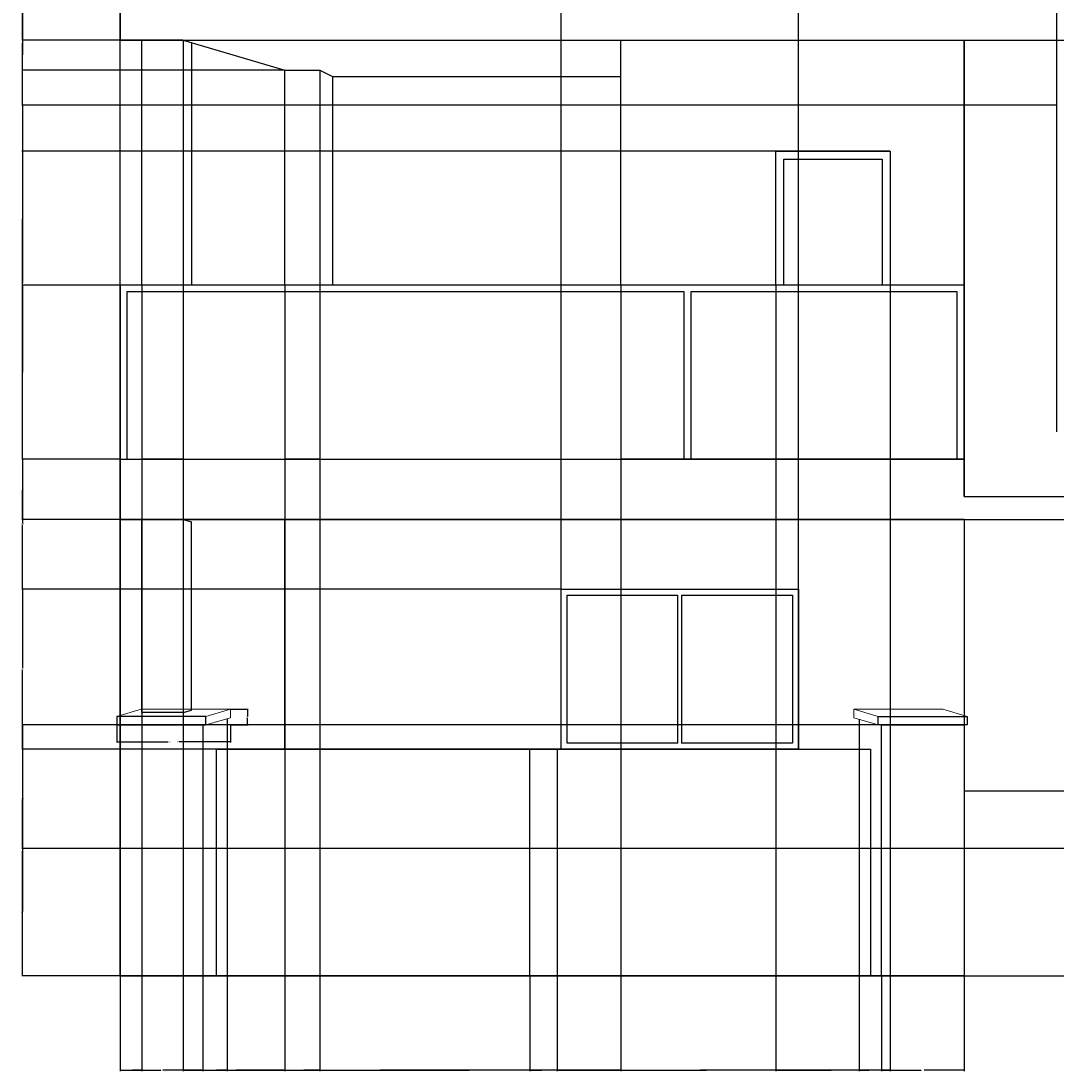
# Model space of a CAD drawing. Units: feet. Extents: x 2926 to 4178, y 965 to 1469.
# Tile 7 of 9: x 3641 to 3913, y 965 to 1241. Entities that reach past the tile are written whole.
import ezdxf

# ---------------------------------------------------------------- set-up
doc = ezdxf.new("R2010")
doc.units = ezdxf.units.FT
for name, color, linetype, lineweight in [('A-ANNO-DIMS', 2, 'Continuous', 18), ('A-ELEV', 7, 'Continuous', 25), ('A-ELEV-DETL', 8, 'Continuous', 18)]:
    doc.layers.add(name, color=color, linetype=linetype, lineweight=lineweight)
doc.styles.get("Standard").update_dxf_attribs({"font": 'arial.ttf'})
doc.dimstyles.get("Standard").update_dxf_attribs({"dimtxt": 0.18, "dimasz": 0.18, "dimexe": 0.18, "dimexo": 0.0625, "dimgap": 0.09, "dimtad": 0, "dimtih": 1, "dimtoh": 1, "dimdec": 1, "dimzin": 0, "dimdsep": 46, "dimlunit": 3, "dimtxsty": 'Standard', "dimcen": 0.09, "dimadec": 0, "dimazin": 0, "dimtfac": 1, "dimtdec": 1, "dimtofl": 0, "dimtmove": 0, "dimatfit": 3, "dimfxl": 1, "dimtolj": 1, "dimtzin": 0, "dimarcsym": 0})

# ---------------------------------------------------------------- blocks, each defined once
blk = doc.blocks.new('PILLAR-CAP-B')
for p, q in [((0, 2.25), (6.42, 4.14)), ((29.85, 4.14), (6.42, 4.14)), ((23.43, 2.25), (29.85, 4.14)), ((29.85, 1.89), (29.85, 4.14)), ((23.43, 0), (29.85, 1.89))]:
    blk.add_line(p, q)
blk = doc.blocks.new('*D8')
at = {"layer": 'A-ANNO-DIMS', "color": 0, "lineweight": -2, "transparency": 16777216}
for p, q in [((3666.26, 1056.26), (3666.26, 1051.66)), ((3696.11, 1056.26), (3696.11, 1051.66)), ((3666.44, 1051.84), (3679.78, 1051.84)), ((3695.93, 1051.84), (3682.59, 1051.84))]:
    blk.add_line(p, q, dxfattribs=at)
at = {"layer": 'A-ANNO-DIMS', "color": 0, "transparency": 16777216}
for points in [[(3666.44, 1051.87), (3666.44, 1051.81), (3666.26, 1051.84)], [(3695.93, 1051.87), (3695.93, 1051.81), (3696.11, 1051.84)]]:
    blk.add_solid(points, dxfattribs=at)
at = {"layer": 'Defpoints', "color": 0, "transparency": 16777216}
for p in [(3666.26, 1056.32), (3696.11, 1056.32), (3696.11, 1051.84)]:
    blk.add_point(p, dxfattribs=at)
at = {"layer": 'A-ANNO-DIMS', "color": 0, "transparency": 16777216, "insert": (3681.19, 1051.84), "char_height": 0.18, "attachment_point": 5}
blk.add_mtext('\\A1;PILLAR CAP B 30 TYP.', dxfattribs=at)
blk = doc.blocks.new('*D9')
at = {"layer": 'A-ANNO-DIMS', "color": 0, "lineweight": -2, "transparency": 16777216}
for p, q in [((3696.17, 1060.46), (3700.77, 1060.46)), ((3700.59, 1060.28), (3700.59, 1058.57)), ((3700.59, 1056.5), (3700.59, 1058.21)), ((3696.17, 1056.32), (3700.77, 1056.32))]:
    blk.add_line(p, q, dxfattribs=at)
at = {"layer": 'A-ANNO-DIMS', "color": 0, "transparency": 16777216}
for points in [[(3700.56, 1060.28), (3700.62, 1060.28), (3700.59, 1060.46)], [(3700.56, 1056.5), (3700.62, 1056.5), (3700.59, 1056.32)]]:
    blk.add_solid(points, dxfattribs=at)
at = {"layer": 'Defpoints', "color": 0, "transparency": 16777216}
for p in [(3696.11, 1060.46), (3700.59, 1060.46), (3696.11, 1056.32)]:
    blk.add_point(p, dxfattribs=at)
at = {"layer": 'A-ANNO-DIMS', "color": 0, "transparency": 16777216, "insert": (3700.59, 1058.39), "char_height": 0.18, "attachment_point": 5}
blk.add_mtext('\\A1;4 TYP.', dxfattribs=at)
blk = doc.blocks.new('*D76')
at = {"layer": 'A-ANNO-DIMS', "color": 0, "lineweight": -2, "transparency": 16777216}
for p, q in [((4050.56, 1023.86), (3641.28, 1023.86)), ((3641.46, 1023.68), (3641.46, 1007.27)), ((3641.46, 990.5), (3641.46, 1006.91)), ((3667.05, 990.32), (3641.28, 990.32))]:
    blk.add_line(p, q, dxfattribs=at)
at = {"layer": 'A-ANNO-DIMS', "color": 0, "transparency": 16777216}
for points in [[(3641.43, 1023.68), (3641.49, 1023.68), (3641.46, 1023.86)], [(3641.43, 990.5), (3641.49, 990.5), (3641.46, 990.32)]]:
    blk.add_solid(points, dxfattribs=at)
at = {"layer": 'Defpoints', "color": 0, "transparency": 16777216}
for p in [(3641.46, 1023.86), (4050.62, 1023.86), (3667.11, 990.32)]:
    blk.add_point(p, dxfattribs=at)
at = {"layer": 'A-ANNO-DIMS', "color": 0, "transparency": 16777216, "insert": (3641.46, 1007.09), "char_height": 0.18, "attachment_point": 5}
blk.add_mtext('\\A1;33.53', dxfattribs=at)
blk = doc.blocks.new('*D77')
at = {"layer": 'A-ANNO-DIMS', "color": 0, "lineweight": -2, "transparency": 16777216}
for p, q in [((3782.96, 1049.98), (3641.28, 1049.98)), ((3641.46, 1049.8), (3641.46, 1037.1)), ((3641.46, 1024.04), (3641.46, 1036.74)), ((4050.56, 1023.86), (3641.28, 1023.86))]:
    blk.add_line(p, q, dxfattribs=at)
at = {"layer": 'A-ANNO-DIMS', "color": 0, "transparency": 16777216}
for points in [[(3641.43, 1049.8), (3641.49, 1049.8), (3641.46, 1049.98)], [(3641.43, 1024.04), (3641.49, 1024.04), (3641.46, 1023.86)]]:
    blk.add_solid(points, dxfattribs=at)
at = {"layer": 'Defpoints', "color": 0, "transparency": 16777216}
for p in [(3641.46, 1049.98), (3783.02, 1049.98), (4050.62, 1023.86)]:
    blk.add_point(p, dxfattribs=at)
at = {"layer": 'A-ANNO-DIMS', "color": 0, "transparency": 16777216, "insert": (3641.46, 1036.92), "char_height": 0.18, "attachment_point": 5}
blk.add_mtext('\\A1;26.13', dxfattribs=at)
blk = doc.blocks.new('*D78')
at = {"layer": 'A-ANNO-DIMS', "color": 0, "lineweight": -2, "transparency": 16777216}
for p, q in [((3782.96, 1092.04), (3641.28, 1092.04)), ((3641.46, 1091.86), (3641.46, 1071.2)), ((3641.46, 1050.16), (3641.46, 1070.83)), ((3782.96, 1049.98), (3641.28, 1049.98))]:
    blk.add_line(p, q, dxfattribs=at)
at = {"layer": 'A-ANNO-DIMS', "color": 0, "transparency": 16777216}
for points in [[(3641.43, 1091.86), (3641.49, 1091.86), (3641.46, 1092.04)], [(3641.43, 1050.16), (3641.49, 1050.16), (3641.46, 1049.98)]]:
    blk.add_solid(points, dxfattribs=at)
at = {"layer": 'Defpoints', "color": 0, "transparency": 16777216}
for p in [(3641.46, 1092.04), (3783.02, 1092.04), (3783.02, 1049.98)]:
    blk.add_point(p, dxfattribs=at)
at = {"layer": 'A-ANNO-DIMS', "color": 0, "transparency": 16777216, "insert": (3641.46, 1071.01), "char_height": 0.18, "attachment_point": 5}
blk.add_mtext('\\A1;42.06', dxfattribs=at)
blk = doc.blocks.new('*D79')
at = {"layer": 'A-ANNO-DIMS', "color": 0, "lineweight": -2, "transparency": 16777216}
for p, q in [((3667.05, 1126.14), (3641.28, 1126.14)), ((3641.46, 1125.96), (3641.46, 1109.27)), ((3641.46, 1092.22), (3641.46, 1108.91)), ((3782.96, 1092.04), (3641.28, 1092.04))]:
    blk.add_line(p, q, dxfattribs=at)
at = {"layer": 'A-ANNO-DIMS', "color": 0, "transparency": 16777216}
for points in [[(3641.43, 1125.96), (3641.49, 1125.96), (3641.46, 1126.14)], [(3641.43, 1092.22), (3641.49, 1092.22), (3641.46, 1092.04)]]:
    blk.add_solid(points, dxfattribs=at)
at = {"layer": 'Defpoints', "color": 0, "transparency": 16777216}
for p in [(3641.46, 1126.14), (3667.11, 1126.14), (3783.02, 1092.04)]:
    blk.add_point(p, dxfattribs=at)
at = {"layer": 'A-ANNO-DIMS', "color": 0, "transparency": 16777216, "insert": (3641.46, 1109.09), "char_height": 0.18, "attachment_point": 5}
blk.add_mtext('\\A1;34.095', dxfattribs=at)
blk = doc.blocks.new('*D80')
at = {"layer": 'A-ANNO-DIMS', "color": 0, "lineweight": -2, "transparency": 16777216}
for p, q in [((3913.29, 1219.22), (3641.28, 1219.22)), ((3641.46, 1219.04), (3641.46, 1172.86)), ((3641.46, 1126.32), (3641.46, 1172.5)), ((3667.05, 1126.14), (3641.28, 1126.14))]:
    blk.add_line(p, q, dxfattribs=at)
at = {"layer": 'A-ANNO-DIMS', "color": 0, "transparency": 16777216}
for points in [[(3641.43, 1219.04), (3641.49, 1219.04), (3641.46, 1219.22)], [(3641.43, 1126.32), (3641.49, 1126.32), (3641.46, 1126.14)]]:
    blk.add_solid(points, dxfattribs=at)
at = {"layer": 'Defpoints', "color": 0, "transparency": 16777216}
for p in [(3641.46, 1219.22), (3913.35, 1219.22), (3667.11, 1126.14)]:
    blk.add_point(p, dxfattribs=at)
at = {"layer": 'A-ANNO-DIMS', "color": 0, "transparency": 16777216, "insert": (3641.46, 1172.68), "char_height": 0.18, "attachment_point": 5}
blk.add_mtext('\\A1;93.08', dxfattribs=at)
blk = doc.blocks.new('*D81')
at = {"layer": 'A-ANNO-DIMS', "color": 0, "lineweight": -2, "transparency": 16777216}
for p, q in [((3667.05, 1252.14), (3641.28, 1252.14)), ((3641.46, 1251.96), (3641.46, 1235.86)), ((3641.46, 1219.4), (3641.46, 1235.5)), ((3913.29, 1219.22), (3641.28, 1219.22))]:
    blk.add_line(p, q, dxfattribs=at)
at = {"layer": 'A-ANNO-DIMS', "color": 0, "transparency": 16777216}
for points in [[(3641.43, 1251.96), (3641.49, 1251.96), (3641.46, 1252.14)], [(3641.43, 1219.4), (3641.49, 1219.4), (3641.46, 1219.22)]]:
    blk.add_solid(points, dxfattribs=at)
at = {"layer": 'Defpoints', "color": 0, "transparency": 16777216}
for p in [(3641.46, 1252.14), (3667.11, 1252.14), (3913.35, 1219.22)]:
    blk.add_point(p, dxfattribs=at)
at = {"layer": 'A-ANNO-DIMS', "color": 0, "transparency": 16777216, "insert": (3641.46, 1235.68), "char_height": 0.18, "attachment_point": 5}
blk.add_mtext('\\A1;32.92', dxfattribs=at)
blk = doc.blocks.new('*D86')
at = {"layer": 'A-ANNO-DIMS', "color": 0, "lineweight": -2, "transparency": 16777216}
for p, q in [((3667.11, 1056.38), (3667.11, 1468.62)), ((3667.29, 1468.44), (3724.68, 1468.44)), ((3782.84, 1468.44), (3725.45, 1468.44)), ((3783.02, 1050.05), (3783.02, 1468.62))]:
    blk.add_line(p, q, dxfattribs=at)
at = {"layer": 'A-ANNO-DIMS', "color": 0, "transparency": 16777216}
for points in [[(3667.29, 1468.47), (3667.29, 1468.41), (3667.11, 1468.44)], [(3782.84, 1468.47), (3782.84, 1468.41), (3783.02, 1468.44)]]:
    blk.add_solid(points, dxfattribs=at)
at = {"layer": 'Defpoints', "color": 0, "transparency": 16777216}
for p in [(3783.02, 1468.44), (3667.11, 1056.32), (3783.02, 1049.98)]:
    blk.add_point(p, dxfattribs=at)
at = {"layer": 'A-ANNO-DIMS', "color": 0, "transparency": 16777216, "insert": (3725.07, 1468.44), "char_height": 0.18, "attachment_point": 5}
blk.add_mtext('\\A1;115.9', dxfattribs=at)
blk = doc.blocks.new('*D87')
at = {"layer": 'A-ANNO-DIMS', "color": 0, "lineweight": -2, "transparency": 16777216}
for p, q in [((3783.02, 1050.05), (3783.02, 1468.62)), ((3783.2, 1468.44), (3813.82, 1468.44)), ((3845.22, 1468.44), (3814.61, 1468.44)), ((3845.4, 1050.05), (3845.4, 1468.62))]:
    blk.add_line(p, q, dxfattribs=at)
at = {"layer": 'A-ANNO-DIMS', "color": 0, "transparency": 16777216}
for points in [[(3783.2, 1468.47), (3783.2, 1468.41), (3783.02, 1468.44)], [(3845.22, 1468.47), (3845.22, 1468.41), (3845.4, 1468.44)]]:
    blk.add_solid(points, dxfattribs=at)
at = {"layer": 'Defpoints', "color": 0, "transparency": 16777216}
for p in [(3845.4, 1468.44), (3783.02, 1049.98), (3845.4, 1049.98)]:
    blk.add_point(p, dxfattribs=at)
at = {"layer": 'A-ANNO-DIMS', "color": 0, "transparency": 16777216, "insert": (3814.21, 1468.44), "char_height": 0.18, "attachment_point": 5}
blk.add_mtext('\\A1;62.38', dxfattribs=at)
blk = doc.blocks.new('*D88')
at = {"layer": 'A-ANNO-DIMS', "color": 0, "lineweight": -2, "transparency": 16777216}
for p, q in [((3845.4, 1050.05), (3845.4, 1468.62)), ((3845.58, 1468.44), (3878.98, 1468.44)), ((3913.17, 1468.44), (3879.77, 1468.44)), ((3913.35, 1133.35), (3913.35, 1468.62))]:
    blk.add_line(p, q, dxfattribs=at)
at = {"layer": 'A-ANNO-DIMS', "color": 0, "transparency": 16777216}
for points in [[(3845.58, 1468.47), (3845.58, 1468.41), (3845.4, 1468.44)], [(3913.17, 1468.47), (3913.17, 1468.41), (3913.35, 1468.44)]]:
    blk.add_solid(points, dxfattribs=at)
at = {"layer": 'Defpoints', "color": 0, "transparency": 16777216}
for p in [(3913.35, 1468.44), (3913.35, 1133.29), (3845.4, 1049.98)]:
    blk.add_point(p, dxfattribs=at)
at = {"layer": 'A-ANNO-DIMS', "color": 0, "transparency": 16777216, "insert": (3879.38, 1468.44), "char_height": 0.18, "attachment_point": 5}
blk.add_mtext('\\A1;67.95', dxfattribs=at)
blk = doc.blocks.new('*D89')
at = {"layer": 'A-ANNO-DIMS', "color": 0, "lineweight": -2, "transparency": 16777216}
for p, q in [((3913.35, 1133.35), (3913.35, 1468.62)), ((3913.53, 1468.44), (3936.04, 1468.44)), ((3959.35, 1468.44), (3936.84, 1468.44)), ((3959.53, 1133.35), (3959.53, 1468.62))]:
    blk.add_line(p, q, dxfattribs=at)
at = {"layer": 'A-ANNO-DIMS', "color": 0, "transparency": 16777216}
for points in [[(3913.53, 1468.47), (3913.53, 1468.41), (3913.35, 1468.44)], [(3959.35, 1468.47), (3959.35, 1468.41), (3959.53, 1468.44)]]:
    blk.add_solid(points, dxfattribs=at)
at = {"layer": 'Defpoints', "color": 0, "transparency": 16777216}
for p in [(3959.53, 1468.44), (3913.35, 1133.29), (3959.53, 1133.29)]:
    blk.add_point(p, dxfattribs=at)
at = {"layer": 'A-ANNO-DIMS', "color": 0, "transparency": 16777216, "insert": (3936.44, 1468.44), "char_height": 0.18, "attachment_point": 5}
blk.add_mtext('\\A1;46.18', dxfattribs=at)
blk = doc.blocks.new('*D114')
at = {"layer": 'A-ANNO-DIMS', "color": 0, "lineweight": -2, "transparency": 16777216}
for p, q in [((3667.11, 1171.83), (3667.11, 965.34)), ((3672.82, 1171.83), (3672.82, 965.34)), ((3667.29, 965.52), (3669.58, 965.52)), ((3672.64, 965.52), (3670.36, 965.52))]:
    blk.add_line(p, q, dxfattribs=at)
at = {"layer": 'A-ANNO-DIMS', "color": 0, "transparency": 16777216}
for points in [[(3667.29, 965.55), (3667.29, 965.49), (3667.11, 965.52)], [(3672.64, 965.55), (3672.64, 965.49), (3672.82, 965.52)]]:
    blk.add_solid(points, dxfattribs=at)
at = {"layer": 'Defpoints', "color": 0, "transparency": 16777216}
for p in [(3667.11, 1171.9), (3672.82, 1171.9), (3672.82, 965.52)]:
    blk.add_point(p, dxfattribs=at)
at = {"layer": 'A-ANNO-DIMS', "color": 0, "transparency": 16777216, "insert": (3669.97, 965.52), "char_height": 0.18, "attachment_point": 5}
blk.add_mtext('\\A1;5.712', dxfattribs=at)
blk = doc.blocks.new('*D115')
at = {"layer": 'A-ANNO-DIMS', "color": 0, "lineweight": -2, "transparency": 16777216}
for p, q in [((3672.82, 1171.83), (3672.82, 965.34)), ((3683.7, 1171.83), (3683.7, 965.34)), ((3673, 965.52), (3677.82, 965.52)), ((3683.52, 965.52), (3678.7, 965.52))]:
    blk.add_line(p, q, dxfattribs=at)
at = {"layer": 'A-ANNO-DIMS', "color": 0, "transparency": 16777216}
for points in [[(3673, 965.55), (3673, 965.49), (3672.82, 965.52)], [(3683.52, 965.55), (3683.52, 965.49), (3683.7, 965.52)]]:
    blk.add_solid(points, dxfattribs=at)
at = {"layer": 'Defpoints', "color": 0, "transparency": 16777216}
for p in [(3672.82, 1171.9), (3683.7, 1171.9), (3683.7, 965.52)]:
    blk.add_point(p, dxfattribs=at)
at = {"layer": 'A-ANNO-DIMS', "color": 0, "transparency": 16777216, "insert": (3678.26, 965.52), "char_height": 0.18, "attachment_point": 5}
blk.add_mtext('\\A1;10.871', dxfattribs=at)
blk = doc.blocks.new('*D116')
at = {"layer": 'A-ANNO-DIMS', "color": 0, "lineweight": -2, "transparency": 16777216}
for p, q in [((3683.7, 1171.83), (3683.7, 965.34)), ((3710.38, 1171.83), (3710.38, 965.34)), ((3683.88, 965.52), (3696.57, 965.52)), ((3710.2, 965.52), (3697.5, 965.52))]:
    blk.add_line(p, q, dxfattribs=at)
at = {"layer": 'A-ANNO-DIMS', "color": 0, "transparency": 16777216}
for points in [[(3683.88, 965.55), (3683.88, 965.49), (3683.7, 965.52)], [(3710.2, 965.55), (3710.2, 965.49), (3710.38, 965.52)]]:
    blk.add_solid(points, dxfattribs=at)
at = {"layer": 'Defpoints', "color": 0, "transparency": 16777216}
for p in [(3683.7, 1171.9), (3710.38, 1171.9), (3710.38, 965.52)]:
    blk.add_point(p, dxfattribs=at)
at = {"layer": 'A-ANNO-DIMS', "color": 0, "transparency": 16777216, "insert": (3697.04, 965.52), "char_height": 0.18, "attachment_point": 5}
blk.add_mtext('\\A1;26.685', dxfattribs=at)
blk = doc.blocks.new('*D117')
at = {"layer": 'A-ANNO-DIMS', "color": 0, "lineweight": -2, "transparency": 16777216}
for p, q in [((3710.38, 1171.83), (3710.38, 965.34)), ((3719.64, 1171.83), (3719.64, 965.34)), ((3710.56, 965.52), (3714.62, 965.52)), ((3719.46, 965.52), (3715.4, 965.52))]:
    blk.add_line(p, q, dxfattribs=at)
at = {"layer": 'A-ANNO-DIMS', "color": 0, "transparency": 16777216}
for points in [[(3710.56, 965.55), (3710.56, 965.49), (3710.38, 965.52)], [(3719.46, 965.55), (3719.46, 965.49), (3719.64, 965.52)]]:
    blk.add_solid(points, dxfattribs=at)
at = {"layer": 'Defpoints', "color": 0, "transparency": 16777216}
for p in [(3710.38, 1171.9), (3719.64, 1171.9), (3719.64, 965.52)]:
    blk.add_point(p, dxfattribs=at)
at = {"layer": 'A-ANNO-DIMS', "color": 0, "transparency": 16777216, "insert": (3715.01, 965.52), "char_height": 0.18, "attachment_point": 5}
blk.add_mtext('\\A1;9.257', dxfattribs=at)
blk = doc.blocks.new('*D118')
at = {"layer": 'A-ANNO-DIMS', "color": 0, "lineweight": -2, "transparency": 16777216}
for p, q in [((3719.64, 1171.83), (3719.64, 965.34)), ((3798.74, 1171.83), (3798.74, 965.34)), ((3719.82, 965.52), (3758.88, 965.52)), ((3798.56, 965.52), (3759.5, 965.52))]:
    blk.add_line(p, q, dxfattribs=at)
at = {"layer": 'A-ANNO-DIMS', "color": 0, "transparency": 16777216}
for points in [[(3719.82, 965.55), (3719.82, 965.49), (3719.64, 965.52)], [(3798.56, 965.55), (3798.56, 965.49), (3798.74, 965.52)]]:
    blk.add_solid(points, dxfattribs=at)
at = {"layer": 'Defpoints', "color": 0, "transparency": 16777216}
for p in [(3719.64, 1171.9), (3798.74, 1171.9), (3798.74, 965.52)]:
    blk.add_point(p, dxfattribs=at)
at = {"layer": 'A-ANNO-DIMS', "color": 0, "transparency": 16777216, "insert": (3759.19, 965.52), "char_height": 0.18, "attachment_point": 5}
blk.add_mtext('\\A1;79.1', dxfattribs=at)
blk = doc.blocks.new('*D119')
at = {"layer": 'A-ANNO-DIMS', "color": 0, "lineweight": -2, "transparency": 16777216}
for p, q in [((3798.74, 1171.83), (3798.74, 965.34)), ((3839.47, 1171.83), (3839.47, 965.34)), ((3798.92, 965.52), (3818.71, 965.52)), ((3839.29, 965.52), (3819.5, 965.52))]:
    blk.add_line(p, q, dxfattribs=at)
at = {"layer": 'A-ANNO-DIMS', "color": 0, "transparency": 16777216}
for points in [[(3798.92, 965.55), (3798.92, 965.49), (3798.74, 965.52)], [(3839.29, 965.55), (3839.29, 965.49), (3839.47, 965.52)]]:
    blk.add_solid(points, dxfattribs=at)
at = {"layer": 'Defpoints', "color": 0, "transparency": 16777216}
for p in [(3798.74, 1171.9), (3839.47, 1171.9), (3839.47, 965.52)]:
    blk.add_point(p, dxfattribs=at)
at = {"layer": 'A-ANNO-DIMS', "color": 0, "transparency": 16777216, "insert": (3819.1, 965.52), "char_height": 0.18, "attachment_point": 5}
blk.add_mtext('\\A1;40.73', dxfattribs=at)
blk = doc.blocks.new('*D120')
at = {"layer": 'A-ANNO-DIMS', "color": 0, "lineweight": -2, "transparency": 16777216}
for p, q in [((3839.47, 1171.83), (3839.47, 965.34)), ((3869.48, 1171.83), (3869.48, 965.34)), ((3839.65, 965.52), (3854.01, 965.52)), ((3869.3, 965.52), (3854.94, 965.52))]:
    blk.add_line(p, q, dxfattribs=at)
at = {"layer": 'A-ANNO-DIMS', "color": 0, "transparency": 16777216}
for points in [[(3839.65, 965.55), (3839.65, 965.49), (3839.47, 965.52)], [(3869.3, 965.55), (3869.3, 965.49), (3869.48, 965.52)]]:
    blk.add_solid(points, dxfattribs=at)
at = {"layer": 'Defpoints', "color": 0, "transparency": 16777216}
for p in [(3839.47, 1171.9), (3869.48, 1171.9), (3869.48, 965.52)]:
    blk.add_point(p, dxfattribs=at)
at = {"layer": 'A-ANNO-DIMS', "color": 0, "transparency": 16777216, "insert": (3854.48, 965.52), "char_height": 0.18, "attachment_point": 5}
blk.add_mtext('\\A1;30.015', dxfattribs=at)
blk = doc.blocks.new('*D121')
at = {"layer": 'A-ANNO-DIMS', "color": 0, "lineweight": -2, "transparency": 16777216}
for p, q in [((3869.42, 1207.11), (3641.28, 1207.11)), ((3641.46, 1206.93), (3641.46, 1189.68)), ((3641.46, 1172.08), (3641.46, 1189.32)), ((3869.42, 1171.9), (3641.28, 1171.9))]:
    blk.add_line(p, q, dxfattribs=at)
at = {"layer": 'A-ANNO-DIMS', "color": 0, "transparency": 16777216}
for points in [[(3641.43, 1206.93), (3641.49, 1206.93), (3641.46, 1207.11)], [(3641.43, 1172.08), (3641.49, 1172.08), (3641.46, 1171.9)]]:
    blk.add_solid(points, dxfattribs=at)
at = {"layer": 'Defpoints', "color": 0, "transparency": 16777216}
for p in [(3641.46, 1207.11), (3869.48, 1207.11), (3869.48, 1171.9)]:
    blk.add_point(p, dxfattribs=at)
at = {"layer": 'A-ANNO-DIMS', "color": 0, "transparency": 16777216, "insert": (3641.46, 1189.5), "char_height": 0.18, "attachment_point": 5}
blk.add_mtext('\\A1;35.21', dxfattribs=at)
blk = doc.blocks.new('*D122')
at = {"layer": 'A-ANNO-DIMS', "color": 0, "lineweight": -2, "transparency": 16777216}
for p, q in [((3683.63, 1236.32), (3641.28, 1236.32)), ((3641.46, 1236.14), (3641.46, 1232.58)), ((3641.46, 1228.64), (3641.46, 1232.21)), ((3710.32, 1228.46), (3641.28, 1228.46))]:
    blk.add_line(p, q, dxfattribs=at)
at = {"layer": 'A-ANNO-DIMS', "color": 0, "transparency": 16777216}
for points in [[(3641.43, 1236.14), (3641.49, 1236.14), (3641.46, 1236.32)], [(3641.43, 1228.64), (3641.49, 1228.64), (3641.46, 1228.46)]]:
    blk.add_solid(points, dxfattribs=at)
at = {"layer": 'Defpoints', "color": 0, "transparency": 16777216}
for p in [(3641.46, 1236.32), (3683.7, 1236.32), (3710.38, 1228.46)]:
    blk.add_point(p, dxfattribs=at)
at = {"layer": 'A-ANNO-DIMS', "color": 0, "transparency": 16777216, "insert": (3641.46, 1232.39), "char_height": 0.18, "attachment_point": 5}
blk.add_mtext('\\A1;7.86', dxfattribs=at)
blk = doc.blocks.new('*D123')
at = {"layer": 'A-ANNO-DIMS', "color": 0, "lineweight": -2, "transparency": 16777216}
for p, q in [((3667.05, 1171.9), (3641.28, 1171.9)), ((3641.46, 1171.72), (3641.46, 1149.2)), ((3641.46, 1126.32), (3641.46, 1148.84)), ((3667.05, 1126.14), (3641.28, 1126.14))]:
    blk.add_line(p, q, dxfattribs=at)
at = {"layer": 'A-ANNO-DIMS', "color": 0, "transparency": 16777216}
for points in [[(3641.43, 1171.72), (3641.49, 1171.72), (3641.46, 1171.9)], [(3641.43, 1126.32), (3641.49, 1126.32), (3641.46, 1126.14)]]:
    blk.add_solid(points, dxfattribs=at)
at = {"layer": 'Defpoints', "color": 0, "transparency": 16777216}
for p in [(3641.46, 1171.9), (3667.11, 1171.9), (3667.11, 1126.14)]:
    blk.add_point(p, dxfattribs=at)
at = {"layer": 'A-ANNO-DIMS', "color": 0, "transparency": 16777216, "insert": (3641.46, 1149.02), "char_height": 0.18, "attachment_point": 5}
blk.add_mtext('\\A1;45.76', dxfattribs=at)
blk = doc.blocks.new('*D124')
at = {"layer": 'A-ANNO-DIMS', "color": 0, "lineweight": -2, "transparency": 16777216}
for p, q in [((3667.05, 1126.14), (3641.28, 1126.14)), ((3641.46, 1125.96), (3641.46, 1118.41)), ((3641.46, 1110.5), (3641.46, 1118.05)), ((3667.05, 1110.32), (3641.28, 1110.32))]:
    blk.add_line(p, q, dxfattribs=at)
at = {"layer": 'A-ANNO-DIMS', "color": 0, "transparency": 16777216}
for points in [[(3641.43, 1125.96), (3641.49, 1125.96), (3641.46, 1126.14)], [(3641.43, 1110.5), (3641.49, 1110.5), (3641.46, 1110.32)]]:
    blk.add_solid(points, dxfattribs=at)
at = {"layer": 'Defpoints', "color": 0, "transparency": 16777216}
for p in [(3641.46, 1126.14), (3667.11, 1126.14), (3667.11, 1110.32)]:
    blk.add_point(p, dxfattribs=at)
at = {"layer": 'A-ANNO-DIMS', "color": 0, "transparency": 16777216, "insert": (3641.46, 1118.23), "char_height": 0.18, "attachment_point": 5}
blk.add_mtext('\\A1;15.814', dxfattribs=at)
blk = doc.blocks.new('*D125')
at = {"layer": 'A-ANNO-DIMS', "color": 0, "lineweight": -2, "transparency": 16777216}
for p, q in [((3667.05, 1252.14), (3641.28, 1252.14)), ((3641.46, 1251.96), (3641.46, 1244.41)), ((3641.46, 1236.5), (3641.46, 1244.05)), ((3667.05, 1236.32), (3641.28, 1236.32))]:
    blk.add_line(p, q, dxfattribs=at)
at = {"layer": 'A-ANNO-DIMS', "color": 0, "transparency": 16777216}
for points in [[(3641.43, 1251.96), (3641.49, 1251.96), (3641.46, 1252.14)], [(3641.43, 1236.5), (3641.49, 1236.5), (3641.46, 1236.32)]]:
    blk.add_solid(points, dxfattribs=at)
at = {"layer": 'Defpoints', "color": 0, "transparency": 16777216}
for p in [(3641.46, 1252.14), (3667.11, 1252.14), (3667.11, 1236.32)]:
    blk.add_point(p, dxfattribs=at)
at = {"layer": 'A-ANNO-DIMS', "color": 0, "transparency": 16777216, "insert": (3641.46, 1244.23), "char_height": 0.18, "attachment_point": 5}
blk.add_mtext('\\A1;15.814', dxfattribs=at)
blk = doc.blocks.new('*D130')
at = {"layer": 'A-ANNO-DIMS', "color": 0, "lineweight": -2, "transparency": 16777216}
for p, q in [((3667.11, 990.26), (3667.11, 965.34)), ((3688.83, 990.26), (3688.83, 965.34)), ((3667.29, 965.52), (3677.58, 965.52)), ((3688.65, 965.52), (3678.37, 965.52))]:
    blk.add_line(p, q, dxfattribs=at)
at = {"layer": 'A-ANNO-DIMS', "color": 0, "transparency": 16777216}
for points in [[(3667.29, 965.55), (3667.29, 965.49), (3667.11, 965.52)], [(3688.65, 965.55), (3688.65, 965.49), (3688.83, 965.52)]]:
    blk.add_solid(points, dxfattribs=at)
at = {"layer": 'Defpoints', "color": 0, "transparency": 16777216}
for p in [(3667.11, 990.32), (3688.83, 990.32), (3688.83, 965.52)]:
    blk.add_point(p, dxfattribs=at)
at = {"layer": 'A-ANNO-DIMS', "color": 0, "transparency": 16777216, "insert": (3677.97, 965.52), "char_height": 0.18, "attachment_point": 5}
blk.add_mtext('\\A1;21.72', dxfattribs=at)
blk = doc.blocks.new('*D131')
at = {"layer": 'A-ANNO-DIMS', "color": 0, "lineweight": -2, "transparency": 16777216}
for p, q in [((3688.83, 990.26), (3688.83, 965.34)), ((3695.24, 990.26), (3695.24, 965.34)), ((3689.01, 965.52), (3691.64, 965.52)), ((3695.06, 965.52), (3692.43, 965.52))]:
    blk.add_line(p, q, dxfattribs=at)
at = {"layer": 'A-ANNO-DIMS', "color": 0, "transparency": 16777216}
for points in [[(3689.01, 965.55), (3689.01, 965.49), (3688.83, 965.52)], [(3695.06, 965.55), (3695.06, 965.49), (3695.24, 965.52)]]:
    blk.add_solid(points, dxfattribs=at)
at = {"layer": 'Defpoints', "color": 0, "transparency": 16777216}
for p in [(3688.83, 990.32), (3695.24, 990.32), (3695.24, 965.52)]:
    blk.add_point(p, dxfattribs=at)
at = {"layer": 'A-ANNO-DIMS', "color": 0, "transparency": 16777216, "insert": (3692.04, 965.52), "char_height": 0.18, "attachment_point": 5}
blk.add_mtext('\\A1;6.406', dxfattribs=at)
blk = doc.blocks.new('*D132')
at = {"layer": 'A-ANNO-DIMS', "color": 0, "lineweight": -2, "transparency": 16777216}
for p, q in [((3695.24, 990.26), (3695.24, 965.34)), ((3774.81, 990.26), (3774.81, 965.34)), ((3695.42, 965.52), (3734.63, 965.52)), ((3774.63, 965.52), (3735.42, 965.52))]:
    blk.add_line(p, q, dxfattribs=at)
at = {"layer": 'A-ANNO-DIMS', "color": 0, "transparency": 16777216}
for points in [[(3695.42, 965.55), (3695.42, 965.49), (3695.24, 965.52)], [(3774.63, 965.55), (3774.63, 965.49), (3774.81, 965.52)]]:
    blk.add_solid(points, dxfattribs=at)
at = {"layer": 'Defpoints', "color": 0, "transparency": 16777216}
for p in [(3695.24, 990.32), (3774.81, 990.32), (3774.81, 965.52)]:
    blk.add_point(p, dxfattribs=at)
at = {"layer": 'A-ANNO-DIMS', "color": 0, "transparency": 16777216, "insert": (3735.03, 965.52), "char_height": 0.18, "attachment_point": 5}
blk.add_mtext('\\A1;79.57', dxfattribs=at)
blk = doc.blocks.new('*D133')
at = {"layer": 'A-ANNO-DIMS', "color": 0, "lineweight": -2, "transparency": 16777216}
for p, q in [((3774.81, 990.26), (3774.81, 965.34)), ((3781.98, 990.26), (3781.98, 965.34)), ((3774.99, 965.52), (3778, 965.52)), ((3781.8, 965.52), (3778.79, 965.52))]:
    blk.add_line(p, q, dxfattribs=at)
at = {"layer": 'A-ANNO-DIMS', "color": 0, "transparency": 16777216}
for points in [[(3774.99, 965.55), (3774.99, 965.49), (3774.81, 965.52)], [(3781.8, 965.55), (3781.8, 965.49), (3781.98, 965.52)]]:
    blk.add_solid(points, dxfattribs=at)
at = {"layer": 'Defpoints', "color": 0, "transparency": 16777216}
for p in [(3774.81, 990.32), (3781.98, 990.32), (3781.98, 965.52)]:
    blk.add_point(p, dxfattribs=at)
at = {"layer": 'A-ANNO-DIMS', "color": 0, "transparency": 16777216, "insert": (3778.4, 965.52), "char_height": 0.18, "attachment_point": 5}
blk.add_mtext('\\A1;7.169', dxfattribs=at)
blk = doc.blocks.new('*D134')
at = {"layer": 'A-ANNO-DIMS', "color": 0, "lineweight": -2, "transparency": 16777216}
for p, q in [((3781.98, 990.26), (3781.98, 965.34)), ((3861.36, 990.26), (3861.36, 965.34)), ((3782.16, 965.52), (3821.28, 965.52)), ((3861.18, 965.52), (3822.06, 965.52))]:
    blk.add_line(p, q, dxfattribs=at)
at = {"layer": 'A-ANNO-DIMS', "color": 0, "transparency": 16777216}
for points in [[(3782.16, 965.55), (3782.16, 965.49), (3781.98, 965.52)], [(3861.18, 965.55), (3861.18, 965.49), (3861.36, 965.52)]]:
    blk.add_solid(points, dxfattribs=at)
at = {"layer": 'Defpoints', "color": 0, "transparency": 16777216}
for p in [(3781.98, 990.32), (3861.36, 990.32), (3861.36, 965.52)]:
    blk.add_point(p, dxfattribs=at)
at = {"layer": 'A-ANNO-DIMS', "color": 0, "transparency": 16777216, "insert": (3821.67, 965.52), "char_height": 0.18, "attachment_point": 5}
blk.add_mtext('\\A1;79.38', dxfattribs=at)
blk = doc.blocks.new('*D135')
at = {"layer": 'A-ANNO-DIMS', "color": 0, "lineweight": -2, "transparency": 16777216}
for p, q in [((3861.36, 990.26), (3861.36, 965.34)), ((3867.21, 990.26), (3867.21, 965.34)), ((3861.54, 965.52), (3863.89, 965.52)), ((3867.03, 965.52), (3864.68, 965.52))]:
    blk.add_line(p, q, dxfattribs=at)
at = {"layer": 'A-ANNO-DIMS', "color": 0, "transparency": 16777216}
for points in [[(3861.54, 965.55), (3861.54, 965.49), (3861.36, 965.52)], [(3867.03, 965.55), (3867.03, 965.49), (3867.21, 965.52)]]:
    blk.add_solid(points, dxfattribs=at)
at = {"layer": 'Defpoints', "color": 0, "transparency": 16777216}
for p in [(3861.36, 990.32), (3867.21, 990.32), (3867.21, 965.52)]:
    blk.add_point(p, dxfattribs=at)
at = {"layer": 'A-ANNO-DIMS', "color": 0, "transparency": 16777216, "insert": (3864.28, 965.52), "char_height": 0.18, "attachment_point": 5}
blk.add_mtext('\\A1;5.849', dxfattribs=at)
blk = doc.blocks.new('*D136')
at = {"layer": 'A-ANNO-DIMS', "color": 0, "lineweight": -2, "transparency": 16777216}
for p, q in [((3867.21, 990.26), (3867.21, 965.34)), ((3888.93, 990.26), (3888.93, 965.34)), ((3867.39, 965.52), (3877.67, 965.52)), ((3888.75, 965.52), (3878.46, 965.52))]:
    blk.add_line(p, q, dxfattribs=at)
at = {"layer": 'A-ANNO-DIMS', "color": 0, "transparency": 16777216}
for points in [[(3867.39, 965.55), (3867.39, 965.49), (3867.21, 965.52)], [(3888.75, 965.55), (3888.75, 965.49), (3888.93, 965.52)]]:
    blk.add_solid(points, dxfattribs=at)
at = {"layer": 'Defpoints', "color": 0, "transparency": 16777216}
for p in [(3867.21, 990.32), (3888.93, 990.32), (3888.93, 965.52)]:
    blk.add_point(p, dxfattribs=at)
at = {"layer": 'A-ANNO-DIMS', "color": 0, "transparency": 16777216, "insert": (3878.07, 965.52), "char_height": 0.18, "attachment_point": 5}
blk.add_mtext('\\A1;21.72', dxfattribs=at)
blk = doc.blocks.new('*D137')
at = {"layer": 'A-ANNO-DIMS', "color": 0, "lineweight": -2, "transparency": 16777216}
for p, q in [((3888.86, 1056.32), (3641.28, 1056.32)), ((3641.46, 1056.14), (3641.46, 1023.5)), ((3641.46, 990.5), (3641.46, 1023.14)), ((3888.86, 990.32), (3641.28, 990.32))]:
    blk.add_line(p, q, dxfattribs=at)
at = {"layer": 'A-ANNO-DIMS', "color": 0, "transparency": 16777216}
for points in [[(3641.43, 1056.14), (3641.49, 1056.14), (3641.46, 1056.32)], [(3641.43, 990.5), (3641.49, 990.5), (3641.46, 990.32)]]:
    blk.add_solid(points, dxfattribs=at)
at = {"layer": 'Defpoints', "color": 0, "transparency": 16777216}
for p in [(3641.46, 1056.32), (3888.93, 1056.32), (3888.93, 990.32)]:
    blk.add_point(p, dxfattribs=at)
at = {"layer": 'A-ANNO-DIMS', "color": 0, "transparency": 16777216, "insert": (3641.46, 1023.32), "char_height": 0.18, "attachment_point": 5}
blk.add_mtext('\\A1;66', dxfattribs=at)

msp = doc.modelspace()

# ---------------------------------------------------------------- linework, layer by layer
at = {"layer": 'A-ELEV'}
for p, q in [((3667.1119, 1236.3246), (3667.1119, 1298.3338)), ((3667.1119, 1236.3246), (3988.3089, 1236.3246)), ((3683.6953, 1236.3246), (3710.3805, 1228.4641)), ((3685.9079, 1235.6728), (3685.9079, 1171.8963)), ((3888.9271, 1116.3246), (3888.9271, 1236.3246)), ((3719.6377, 1228.4641), (3722.9903, 1226.8042)), ((3722.9903, 1226.8042), (3722.9903, 1171.8963)), ((3722.9903, 1226.8042), (3798.7415, 1226.8042)), ((3667.1119, 1110.3246), (3667.1119, 1126.1389)), ((3888.9271, 1116.3246), (3988.3089, 1116.3246)), ((3667.1119, 1110.3246), (4004.1232, 1110.3246)), ((3683.6953, 1110.3246), (3685.9079, 1109.6728)), ((3685.9079, 1060.2025), (3685.9079, 1109.6728)), ((3888.9271, 1110.3246), (3888.9271, 990.3246)), ((3683.6953, 1059.5508), (3685.9079, 1060.2025)), ((3695.2396, 1057.9557), (3695.2396, 990.3246)), ((3861.357, 1057.7915), (3861.357, 990.3246)), ((3667.1119, 990.3246), (3667.1119, 1056.3197)), ((4004.1232, 1038.9216), (3888.9271, 1038.9216)), ((3667.1119, 990.3246), (4147.1119, 990.3246))]:
    msp.add_line(p, q, dxfattribs=at)
for points in [[(4004.1232, 1236.3246), (4004.1232, 1252.1389), (3667.1119, 1252.1389), (3667.1119, 1236.3246), (3988.3089, 1236.3246)], [(3672.824, 1171.8963), (3672.824, 1236.3246), (3683.6953, 1236.3246), (3683.6953, 1171.8963)], [(3798.7415, 1171.8963), (3798.7415, 1236.3246), (3888.9271, 1236.3246), (3888.9271, 1126.1389), (3798.7415, 1126.1389)], [(3710.3805, 1171.8963), (3710.3805, 1228.4641), (3719.6377, 1228.4641), (3719.6377, 1171.8963)], [(3839.4676, 1171.8963), (3839.4676, 1207.1083), (3869.483, 1207.1083), (3869.483, 1171.8963)], [(3841.5785, 1171.8963), (3841.5785, 1204.9974), (3867.3721, 1204.9974), (3867.3721, 1171.8963)], [(3668.9802, 1171.8963), (3667.1119, 1171.8963), (3667.1119, 1126.1389), (3668.9802, 1126.1389), (3668.9802, 1170.2176)], [(3888.9271, 1170.2176), (3888.9271, 1171.8963), (3667.1119, 1171.8963), (3667.1119, 1170.2176)], [(3887.0589, 1170.2176), (3887.0589, 1126.1389), (3888.9271, 1126.1389), (3888.9271, 1171.8963), (3887.0589, 1171.8963)], [(3668.9802, 1170.2176), (3815.3002, 1170.2176)], [(3815.3002, 1170.2176), (3815.3002, 1126.1389), (3817.1685, 1126.1389), (3817.1685, 1170.2176)], [(3817.1685, 1170.2176), (3887.0589, 1170.2176)], [(3888.9271, 1110.3246), (3667.1119, 1110.3246), (3667.1119, 1126.1389), (3888.9271, 1126.1389), (3888.9271, 1116.3246)], [(3683.6953, 1126.1389), (3672.824, 1126.1389)], [(3719.6377, 1126.1389), (3710.3805, 1126.1389)], [(3869.483, 1126.1389), (3839.4676, 1126.1389)], [(3813.7117, 1051.5643), (3784.6031, 1051.5643), (3784.6031, 1090.4638), (3813.7117, 1090.4638)], [(3813.7117, 1051.5643), (3813.7117, 1090.4638)], [(3814.7099, 1090.4638), (3843.8186, 1090.4638), (3843.8186, 1051.5643), (3814.7099, 1051.5643)], [(3814.7099, 1090.4638), (3814.7099, 1051.5643)]]:
    msp.add_lwpolyline(points, dxfattribs=at)
for points in [[(3672.824, 1110.3246), (3683.6953, 1110.3246), (3683.6953, 1059.5508), (3672.824, 1059.5508)], [(3710.3805, 1110.3246), (3719.6377, 1110.3246), (3719.6377, 1049.9841), (3710.3805, 1049.9841)], [(3783.0229, 1092.0439), (3845.3987, 1092.0439), (3845.3987, 1049.9841), (3783.0229, 1049.9841)], [(3666.2599, 1056.3197), (3689.6856, 1056.3197), (3689.6856, 1058.5694), (3666.2599, 1058.5694)], [(3889.7791, 1056.3197), (3866.3535, 1056.3197), (3866.3535, 1058.5694), (3889.7791, 1058.5694)], [(3688.8336, 990.3246), (3667.1119, 990.3246), (3667.1119, 1056.3197), (3688.8336, 1056.3197)], [(3888.9271, 990.3246), (3867.2055, 990.3246), (3867.2055, 1056.3197), (3888.9271, 1056.3197)], [(3692.4384, 1049.9841), (3864.355, 1049.9841), (3864.355, 990.3246), (3692.4384, 990.3246)], [(3774.8122, 1049.9841), (3781.9813, 1049.9841), (3781.9813, 990.3246), (3774.8122, 990.3246)]]:
    msp.add_lwpolyline(points, close=True, dxfattribs=at)

# ---------------------------------------------------------------- block references
at = {"layer": 'A-ELEV-DETL'}
msp.add_blockref('PILLAR-CAP-B', (3666.26, 1056.32), dxfattribs=at)
at = {"layer": 'A-ELEV-DETL', "extrusion": (0, 0, -1), "zscale": -1}
msp.add_blockref('PILLAR-CAP-B', (-3889.7791, 1056.32), dxfattribs=at)

# ---------------------------------------------------------------- dimensions: what is measured, and where the dimension line sits
at = {"layer": 'A-ANNO-DIMS'}
for base, p1, p2, override, picture, middle in [((3783.0229, 1468.4445), (3667.1119, 1056.3197), (3783.0229, 1049.9841), {"dimdec": 1, "dimlfac": 1, "dimrnd": 0, "dimzin": 0, "dimdsep": 46, "dimlunit": 2}, '*D86', (3725.0674, 1468.4445)), ((3845.3987, 1468.4445), (3783.0229, 1049.9841), (3845.3987, 1049.9841), {"dimdec": 2, "dimlfac": 1, "dimrnd": 0, "dimzin": 0, "dimdsep": 46, "dimlunit": 2}, '*D87', (3814.2108, 1468.4445)), ((3913.3516, 1468.4445), (3845.3987, 1049.9841), (3913.3516, 1133.2879), {"dimdec": 2, "dimlfac": 1, "dimrnd": 0, "dimzin": 0, "dimdsep": 46, "dimlunit": 2}, '*D88', (3879.3752, 1468.4445)), ((3959.5291, 1468.4445), (3913.3516, 1133.2879), (3959.5291, 1133.2879), {"dimdec": 2, "dimlfac": 1, "dimrnd": 0, "dimzin": 0, "dimdsep": 46, "dimlunit": 2}, '*D89', (3936.4404, 1468.4445)), ((3672.824, 965.5246), (3667.1119, 1171.8963), (3672.824, 1171.8963), {"dimdec": 3, "dimlfac": 1, "dimrnd": 0, "dimzin": 0, "dimdsep": 46, "dimlunit": 2}, '*D114', (3669.968, 965.5246)), ((3683.6953, 965.5246), (3672.824, 1171.8963), (3683.6953, 1171.8963), {"dimdec": 3, "dimlfac": 1, "dimrnd": 0, "dimzin": 0, "dimdsep": 46, "dimlunit": 2}, '*D115', (3678.2597, 965.5246)), ((3710.3805, 965.5246), (3683.6953, 1171.8963), (3710.3805, 1171.8963), {"dimdec": 3, "dimlfac": 1, "dimrnd": 0, "dimzin": 0, "dimdsep": 46, "dimlunit": 2}, '*D116', (3697.0379, 965.5246)), ((3719.6377, 965.5246), (3710.3805, 1171.8963), (3719.6377, 1171.8963), {"dimdec": 3, "dimlfac": 1, "dimrnd": 0, "dimzin": 0, "dimdsep": 46, "dimlunit": 2}, '*D117', (3715.0091, 965.5246)), ((3798.7415, 965.5246), (3719.6377, 1171.8963), (3798.7415, 1171.8963), {"dimdec": 1, "dimlfac": 1, "dimrnd": 0, "dimzin": 0, "dimdsep": 46, "dimlunit": 2}, '*D118', (3759.1896, 965.5246)), ((3839.4676, 965.5246), (3798.7415, 1171.8963), (3839.4676, 1171.8963), {"dimdec": 2, "dimlfac": 1, "dimrnd": 0, "dimzin": 0, "dimdsep": 46, "dimlunit": 2}, '*D119', (3819.1046, 965.5246)), ((3869.483, 965.5246), (3839.4676, 1171.8963), (3869.483, 1171.8963), {"dimdec": 3, "dimlfac": 1, "dimrnd": 0, "dimzin": 0, "dimdsep": 46, "dimlunit": 2}, '*D120', (3854.4753, 965.5246)), ((3688.8336, 965.5246), (3667.1119, 990.3246), (3688.8336, 990.3246), {"dimdec": 2, "dimlfac": 1, "dimrnd": 0, "dimzin": 0, "dimdsep": 46, "dimlunit": 2}, '*D130', (3677.9728, 965.5246)), ((3695.2396, 965.5246), (3688.8336, 990.3246), (3695.2396, 990.3246), {"dimdec": 3, "dimlfac": 1, "dimrnd": 0, "dimzin": 0, "dimdsep": 46, "dimlunit": 2}, '*D131', (3692.0366, 965.5246)), ((3774.8122, 965.5246), (3695.2396, 990.3246), (3774.8122, 990.3246), {"dimdec": 2, "dimlfac": 1, "dimrnd": 0, "dimzin": 0, "dimdsep": 46, "dimlunit": 2}, '*D132', (3735.0259, 965.5246)), ((3781.9813, 965.5246), (3774.8122, 990.3246), (3781.9813, 990.3246), {"dimdec": 3, "dimlfac": 1, "dimrnd": 0, "dimzin": 0, "dimdsep": 46, "dimlunit": 2}, '*D133', (3778.3967, 965.5246)), ((3861.357, 965.5246), (3781.9813, 990.3246), (3861.357, 990.3246), {"dimdec": 2, "dimlfac": 1, "dimrnd": 0, "dimzin": 0, "dimdsep": 46, "dimlunit": 2}, '*D134', (3821.6691, 965.5246)), ((3867.20549, 965.52457), (3861.35698, 990.32457), (3867.20549, 990.32457), {"dimdec": 3, "dimlfac": 1, "dimrnd": 0, "dimzin": 0, "dimdsep": 46, "dimlunit": 2}, '*D135', (3864.28124, 965.52457)), ((3888.9271, 965.5246), (3867.2055, 990.3246), (3888.9271, 990.3246), {"dimdec": 2, "dimlfac": 1, "dimrnd": 0, "dimzin": 0, "dimdsep": 46, "dimlunit": 2}, '*D136', (3878.0663, 965.5246))]:
    dim = msp.add_linear_dim(base=base, p1=p1, p2=p2, dimstyle='Standard', override=override, dxfattribs=at)
    dim.commit()
    dim.dimension.update_dxf_attribs({"geometry": picture, "text_midpoint": middle})
for base, p1, p2, override, picture, middle in [((3641.4599, 1252.1389), (3667.1119, 1236.3246), (3667.1119, 1252.1389), {"dimdec": 3, "dimlfac": 1, "dimrnd": 0, "dimzin": 0, "dimdsep": 46, "dimlunit": 2}, '*D125', (3641.4599, 1244.2317)), ((3641.4599, 1252.1389), (3913.3516, 1219.2195), (3667.1119, 1252.1389), {"dimdec": 2, "dimlfac": 1, "dimrnd": 0, "dimzin": 0, "dimdsep": 46, "dimlunit": 2}, '*D81', (3641.4599, 1235.6792)), ((3641.4599, 1236.3246), (3710.3805, 1228.4641), (3683.6953, 1236.3246), {"dimdec": 2, "dimlfac": 1, "dimrnd": 0, "dimzin": 0, "dimdsep": 46, "dimlunit": 2}, '*D122', (3641.4599, 1232.3943)), ((3641.4599, 1219.2195), (3667.1119, 1126.1389), (3913.3516, 1219.2195), {"dimdec": 2, "dimlfac": 1, "dimrnd": 0, "dimzin": 0, "dimdsep": 46, "dimlunit": 2}, '*D80', (3641.4599, 1172.6792)), ((3641.4599, 1207.1083), (3869.483, 1171.8963), (3869.483, 1207.1083), {"dimdec": 2, "dimlfac": 1, "dimrnd": 0, "dimzin": 0, "dimdsep": 46, "dimlunit": 2}, '*D121', (3641.4599, 1189.5023)), ((3641.4599, 1171.8963), (3667.1119, 1126.1389), (3667.1119, 1171.8963), {"dimdec": 2, "dimlfac": 1, "dimrnd": 0, "dimzin": 0, "dimdsep": 46, "dimlunit": 2}, '*D123', (3641.4599, 1149.0176)), ((3641.4599, 1126.1389), (3783.0229, 1092.0439), (3667.1119, 1126.1389), {"dimdec": 3, "dimlfac": 1, "dimrnd": 0, "dimzin": 0, "dimdsep": 46, "dimlunit": 2}, '*D79', (3641.4599, 1109.0914)), ((3641.4599, 1126.1389), (3667.1119, 1110.3246), (3667.1119, 1126.1389), {"dimdec": 3, "dimlfac": 1, "dimrnd": 0, "dimzin": 0, "dimdsep": 46, "dimlunit": 2}, '*D124', (3641.4599, 1118.2317)), ((3641.4599, 1092.0439), (3783.0229, 1049.9841), (3783.0229, 1092.0439), {"dimdec": 2, "dimlfac": 1, "dimrnd": 0, "dimzin": 0, "dimdsep": 46, "dimlunit": 2}, '*D78', (3641.4599, 1071.014)), ((3641.4599, 1056.3197), (3888.9271, 990.3246), (3888.9271, 1056.3197), {"dimdec": 0, "dimlfac": 1, "dimrnd": 0, "dimzin": 0, "dimdsep": 46, "dimlunit": 2}, '*D137', (3641.4599, 1023.3221)), ((3641.4599, 1049.9841), (4050.6244, 1023.8561), (3783.0229, 1049.9841), {"dimdec": 2, "dimlfac": 1, "dimrnd": 0, "dimzin": 0, "dimdsep": 46, "dimlunit": 2}, '*D77', (3641.4599, 1036.9201)), ((3641.4599, 1023.8561), (3667.1119, 990.3246), (4050.6244, 1023.8561), {"dimdec": 2, "dimlfac": 1, "dimrnd": 0, "dimzin": 0, "dimdsep": 46, "dimlunit": 2}, '*D76', (3641.4599, 1007.0903))]:
    dim = msp.add_linear_dim(base=base, p1=p1, p2=p2, angle=90, dimstyle='Standard', override=override, dxfattribs=at)
    dim.commit()
    dim.dimension.update_dxf_attribs({"geometry": picture, "text_midpoint": middle})
dim = msp.add_linear_dim(base=(3700.5882, 1060.462), p1=(3696.1106, 1056.3197), p2=(3696.1106, 1060.462), angle=90, text='<> TYP.', dimstyle='Standard', override={"dimdec": 0, "dimlfac": 1, "dimrnd": 0, "dimzin": 0, "dimdsep": 46, "dimlunit": 2}, dxfattribs=at)
dim.commit()
dim.dimension.update_dxf_attribs({"geometry": '*D9', "text_midpoint": (3700.5882, 1058.3908)})
dim = msp.add_linear_dim(base=(3696.1106, 1051.8421), p1=(3666.2599, 1056.3197), p2=(3696.1106, 1056.3197), text='PILLAR CAP B <> TYP.', dimstyle='Standard', override={"dimdec": 0, "dimlfac": 1, "dimrnd": 0, "dimzin": 0, "dimdsep": 46, "dimlunit": 2}, dxfattribs=at)
dim.commit()
dim.dimension.update_dxf_attribs({"geometry": '*D8', "text_midpoint": (3681.1852, 1051.8421)})

doc.saveas('drawing.dxf')
